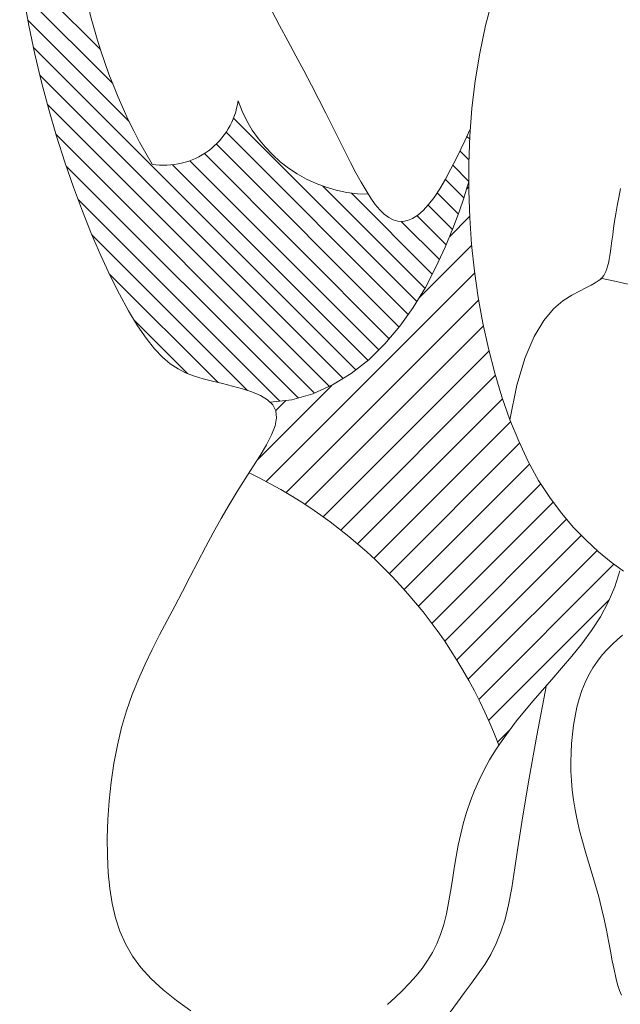
# Model space of a CAD drawing. Units: inches. Extents: x -17 to 1735, y -531 to 60.
# Tile 8 of 27: x 1734.671729 to 1734.673629, y -150.221388 to -150.218274. Entities that reach past the tile are written whole.
import ezdxf

# ---------------------------------------------------------------- set-up
doc = ezdxf.new("R2010")
doc.units = ezdxf.units.IN
doc.header["$MEASUREMENT"] = 0
doc.layers.add('A-FURN', color=242, linetype='Continuous', lineweight=18, true_color=0xcd2027)

# ---------------------------------------------------------------- blocks, each defined once
blk = doc.blocks.new('childrens_room_2')
for p, q in [((70.08834575234098, 54.10698021353749), (70.08185483306764, 54.11347113283994)), ((70.08930673154421, 54.10429042615437), (70.08214777633432, 54.11144938138608)), ((70.08258798463388, 54.10893278750013), (70.08217230242329, 54.11128011434488)), ((70.11988434807748, 54.11121103807676), (70.11928737653537, 54.10893150579653)), ((70.10208583985107, 54.11016166533085), (70.10273900536006, 54.10891733597094)), ((70.0906485886185, 54.10121976091471), (70.08251318732394, 54.10935516215835)), ((70.08306719829444, 54.10662777216789), (70.08258798463388, 54.10893278750013)), ((70.10273900536006, 54.10891733597094), (70.1033990907122, 54.10769144112276)), ((70.11928737653537, 54.10893150579653), (70.11881939316984, 54.1066923617604)), ((70.10887354584295, 54.08126599547398), (70.08295051288908, 54.10718902840603)), ((70.1033990907122, 54.10769144112276), (70.10405456281617, 54.10648398077904)), ((70.08360320534442, 54.10437083808796), (70.08306719829444, 54.10662777216789)), ((70.10405456281617, 54.10648398077904), (70.10469388840605, 54.10529495493978)), ((70.11881939316984, 54.1066923617604), (70.11846210860998, 54.10447341183175)), ((70.10784346914036, 54.08056726393846), (70.08346719220165, 54.10494354092083)), ((70.10469388840605, 54.10529495493978), (70.10530755250832, 54.10412561178095)), ((70.0841892674903, 54.10216775501471), (70.08360320534442, 54.10437083808796)), ((70.10530755250832, 54.10412561178095), (70.10589411355207, 54.10298219213877)), ((70.11846210860998, 54.10447341183175), (70.11819980044268, 54.10225846865654)), ((70.10674630752649, 54.07993561737971), (70.0840715120535, 54.10261041284542)), ((70.09941784066498, 54.10282335800587), (70.0993978207803, 54.10284337791239)), ((70.10589411355207, 54.10298219213877), (70.10645414814238, 54.10187218504001)), ((70.08481864655506, 54.10002429269519), (70.0841892674903, 54.10216775501471)), ((70.10645414814238, 54.10187218504001), (70.10698823294254, 54.10080307951142)), ((70.11819980044268, 54.10225846865654), (70.11802701396985, 54.10004737197454)), ((70.11376654561494, 54.0867458448833), (70.09903804528177, 54.10147434520189)), ((70.10698823294254, 54.10080307951142), (70.10749694461586, 54.09978236455794)), ((70.10555079970393, 54.07940231700052), (70.0847728476033, 54.10018026907204)), ((70.08548460436171, 54.09794622087651), (70.08481864655506, 54.10002429269519)), ((70.11307666940732, 54.08570691289646), (70.09844286601177, 54.10034071627745)), ((70.11762279925054, 54.09966620707422), (70.1178864010831, 54.10023832820883)), ((70.1180167069647, 54.09978376548536), (70.11778412475135, 54.10001634771328)), ((70.1178864010831, 54.10023832820883), (70.118074405425, 54.1006538262431)), ((70.11802701396985, 54.10004737197454), (70.1179408612766, 54.09784396827894)), ((70.11235278042616, 54.08470199369043), (70.09765760974145, 54.09939716433149)), ((70.10749694461586, 54.09978236455794), (70.10798085982563, 54.09881752921359)), ((70.11729604716996, 54.09897629695336), (70.11762279925054, 54.09966620707422)), ((70.11155901827036, 54.08376694762996), (70.09669325274766, 54.09863271315265)), ((70.10798085982563, 54.09881752921359), (70.10844055523515, 54.09791606249058)), ((70.11691859208398, 54.09820743196036), (70.11729604716996, 54.09897629695336)), ((70.11795165449033, 54.0981200097944), (70.11722996820347, 54.0988416960376)), ((70.08618040267496, 54.09593930932027), (70.08548460436171, 54.09794622087651)), ((70.10422052682728, 54.07900378167545), (70.08559420123812, 54.09763010723549)), ((70.10983944662033, 54.08202890289834), (70.09413392528543, 54.09773442420413)), ((70.11072027858928, 54.08287687909473), (70.09553577746149, 54.09806138022253)), ((70.10844055523515, 54.09791606249058), (70.10887660750771, 54.0970854534084)), ((70.11650288117701, 54.09739844620202), (70.11691859208398, 54.09820743196036)), ((70.11793927983265, 54.09640357623579), (70.11665275362203, 54.09769010243912)), ((70.1179408612766, 54.09784396827894), (70.11793845473906, 54.09565210409204)), ((70.10887660750771, 54.0970854534084), (70.10929016996991, 54.09633203883863)), ((70.11606136174989, 54.09658817380699), (70.11650288117701, 54.09739844620202)), ((70.10929016996991, 54.09633203883863), (70.10968470260153, 54.09565754700309)), ((70.11560648104526, 54.09581544887481), (70.11606136174989, 54.09658817380699)), ((70.11754243845238, 54.09507160942888), (70.11604821205722, 54.09656583583132)), ((70.11793922599057, 54.09635456403197), (70.11779819942197, 54.09588022690008)), ((70.08689930331778, 54.09401060992826), (70.08618040267496, 54.09593930932027)), ((70.11441734911524, 54.08782384955561), (70.106220925994, 54.09602027270597)), ((70.11501391657978, 54.08895609029281), (70.10850567942137, 54.09546432743667)), ((70.10968470260153, 54.09565754700309), (70.11006424204562, 54.09506255399032)), ((70.11515068624752, 54.09511910551959), (70.11560648104526, 54.09581544887481)), ((70.11709852587549, 54.09378671381858), (70.11539416219924, 54.09549107745846)), ((70.11779819942197, 54.09588022690008), (70.11753767607618, 54.09505655266406)), ((70.11777364987532, 54.0958026108114), (70.11793880130747, 54.09596776225811)), ((70.11793845473906, 54.09565210409204), (70.11801690650057, 54.09347562589977)), ((70.1301482338563, 54.09583144119682), (70.12999662443647, 54.09511539372619)), ((70.10274766078103, 54.07874783951996), (70.08655132895686, 54.09494417134414)), ((70.11006424204562, 54.09506255399032), (70.1104328248289, 54.09454763587422)), ((70.1104328248289, 54.09454763587422), (70.11079448776903, 54.09411336873603)), ((70.11426916277154, 54.094053744468), (70.11470430205694, 54.09453083342526)), ((70.11662620574819, 54.09253022573688), (70.11466675968725, 54.09448967177599)), ((70.11470430205694, 54.09453083342526), (70.11515068624752, 54.09511910551959)), ((70.11753767607618, 54.09505655266406), (70.11715804838926, 54.0939461216389)), ((70.12999662443647, 54.09511539372619), (70.12986671611318, 54.09443683829744)), ((70.08763456811315, 54.09217230329381), (70.08689930331778, 54.09401060992826)), ((70.11079448776903, 54.09411336873603), (70.11115326739267, 54.09376032865697)), ((70.11115326739267, 54.09376032865697), (70.1115132003429, 54.09348909171098)), ((70.11343146547327, 54.09341698579959), (70.11384498003056, 54.09368380610835)), ((70.11384498003056, 54.09368380610835), (70.11426916277154, 54.094053744468)), ((70.11715804838926, 54.0939461216389), (70.11665970868083, 54.09261151413961)), ((70.12975570048323, 54.09379654006483), (70.12966076914338, 54.09319526417533)), ((70.12986671611318, 54.09443683829744), (70.12975570048323, 54.09379654006483)), ((70.1115132003429, 54.09348909171098), (70.1118783232628, 54.09330023397927)), ((70.1118783232628, 54.09330023397927), (70.11225204811083, 54.09319490761703)), ((70.11225204811083, 54.09319490761703), (70.11263528787416, 54.09317656910428)), ((70.11558285554523, 54.09011595952183), (70.11253988749698, 54.09315892757735)), ((70.11263528787416, 54.09317656910428), (70.11302833085531, 54.0932492509732)), ((70.11302833085531, 54.0932492509732), (70.11343146547327, 54.09341698579959)), ((70.11612163642306, 54.09130598684573), (70.11378349219333, 54.09364413108272)), ((70.11638447265025, 54.09194370757035), (70.11801340944251, 54.09357264436988)), ((70.11801690650057, 54.09347562589977), (70.11817332870444, 54.09131838022443)), ((70.12966076914338, 54.09319526417533), (70.12957911374863, 54.09263377577594)), ((70.08837945888402, 54.09043785216494), (70.08763456811315, 54.09217230329381)), ((70.1001495324995, 54.07961715961431), (70.08766481304659, 54.09210187905268)), ((70.11665970868083, 54.09261151413961), (70.11604304927053, 54.09111531046659)), ((70.12950792589575, 54.09211284002089), (70.12944439723972, 54.09163322204989)), ((70.12957911374863, 54.09263377577594), (70.12950792589575, 54.09211284002089)), ((70.11817332870444, 54.09131838022443), (70.11840483366862, 54.08918421355924)), ((70.12944439723972, 54.09163322204989), (70.12938571937732, 54.09119568702448)), ((70.11393444037415, 54.08702394930736), (70.11817876413582, 54.09126827305448)), ((70.11604304927053, 54.09111531046659), (70.115308462478, 54.08952009093486)), ((70.12932933926234, 54.0908004049765), (70.12927372504376, 54.09044516548459)), ((70.12938571937732, 54.09119568702448), (70.12932933926234, 54.0908004049765)), ((70.08912723745337, 54.08882071929696), (70.08837945888402, 54.09043785216494)), ((70.12915968820337, 54.08984359206664), (70.12909871253535, 54.08959164707488)), ((70.12921760022758, 54.0901271630268), (70.12915968820337, 54.08984359206664)), ((70.12927372504376, 54.09044516548459), (70.12921760022758, 54.0901271630268)), ((70.0977938393585, 54.08024404456813), (70.08904988628231, 54.08898799764433)), ((70.10167231330298, 54.07229209627115), (70.11842493766336, 54.08904472059515)), ((70.115308462478, 54.08952009093486), (70.11445634062287, 54.0878884358521)), ((70.11840483366862, 54.08918421355924), (70.11870853347821, 54.08707697241192)), ((70.12888463820448, 54.08899751263238), (70.12879664265668, 54.08884299603818)), ((70.12896246405901, 54.08917141289425), (70.12888463820448, 54.08899751263238)), ((70.1290333966713, 54.08936852252958), (70.12896246405901, 54.08917141289425)), ((70.12909871253535, 54.08959164707488), (70.1290333966713, 54.08936852252958)), ((70.08987116564415, 54.08733436743062), (70.08912723745337, 54.08882071929696)), ((70.1280974439683, 54.08825043450491), (70.12776946056286, 54.08806403692)), ((70.12835087797023, 54.08841260252524), (70.1280974439683, 54.08825043450491)), ((70.12854303845555, 54.08855946766419), (70.12835087797023, 54.08841260252524)), ((70.12868720136933, 54.08869995660501), (70.12854303845555, 54.08855946766419)), ((70.12879664265668, 54.08884299603818), (70.12868720136933, 54.08869995660501)), ((70.09060450527934, 54.0859922593358), (70.08987116564415, 54.08733436743062)), ((70.11445634062287, 54.0878884358521), (70.11348707602475, 54.08628292553334)), ((70.12683674170287, 54.0875828463308), (70.1262128378253, 54.08725917655686)), ((70.12735365175061, 54.08784448308728), (70.12683674170287, 54.0875828463308)), ((70.12776946056286, 54.08806403692), (70.12735365175061, 54.08784448308728)), ((70.10325632891502, 54.07140638584536), (70.11874183262583, 54.08689188956344)), ((70.11870853347821, 54.08707697241192), (70.11908186135, 54.08500194572702)), ((70.12550558104297, 54.08680943005896), (70.12474599568989, 54.08615853973464)), ((70.1262128378253, 54.08725917655686), (70.12550558104297, 54.08680943005896)), ((70.0913205181237, 54.08480785774594), (70.09060450527934, 54.0859922593358)), ((70.11348707602475, 54.08628292553334), (70.11240187189426, 54.08475982311796)), ((70.12474599568989, 54.08615853973464), (70.12396510610009, 54.08523143845963)), ((70.09534503247006, 54.08096404322572), (70.09104428726597, 54.08526478844436)), ((70.11908186135, 54.08500194572702), (70.11952353368864, 54.08297019219611)), ((70.12396510610009, 54.08523143845963), (70.12319393660756, 54.08395305912421)), ((70.09201246605836, 54.08379462541637), (70.0913205181237, 54.08480785774594)), ((70.10478089296842, 54.07046122392642), (70.11912467337562, 54.08480500434092)), ((70.11240187189426, 54.08475982311796), (70.11120517518023, 54.08335012305764)), ((70.09267649864663, 54.08295993482028), (70.09201246605836, 54.08379462541637)), ((70.12319393660756, 54.08395305912421), (70.12246351148816, 54.08224833462594)), ((70.09332031676198, 54.08228679722964), (70.09267649864663, 54.08295993482028)), ((70.10624785745632, 54.06945846237653), (70.11957188877162, 54.08278249373546)), ((70.11120517518023, 54.08335012305764), (70.10990224378068, 54.08207850265029)), ((70.11952353368864, 54.08297019219611), (70.12003258791404, 54.08099421292575)), ((70.09395450890182, 54.08175213365615), (70.09332031676198, 54.08228679722964)), ((70.10990224378068, 54.08207850265029), (70.1084983354772, 54.08096963918655)), ((70.12246351148816, 54.08224833462594), (70.12180485513412, 54.0800421978551)), ((70.09458966362175, 54.08133286510423), (70.09395450890182, 54.08175213365615)), ((70.09523636953557, 54.08100591256374), (70.09458966362175, 54.08133286510423)), ((70.09590521525709, 54.0807481970391), (70.09523636953557, 54.08100591256374)), ((70.0966067893419, 54.08053663953473), (70.09590521525709, 54.0807481970391)), ((70.0973516802874, 54.08034816104777), (70.0966067893419, 54.08053663953473)), ((70.09814325732762, 54.08016176609675), (70.0973516802874, 54.08034816104777)), ((70.1084983354772, 54.08096963918655), (70.10699870810961, 54.08004820996433)), ((70.10765865067836, 54.06839952964077), (70.12008374557948, 54.08082462454188)), ((70.12003258791404, 54.08099421292575), (70.12060806150433, 54.07908650905159)), ((70.09895601147903, 54.07996479327852), (70.09814325732762, 54.08016176609675)), ((70.09975721443655, 54.07974666471858), (70.09895601147903, 54.07996479327852)), ((70.10051413783688, 54.07949680254245), (70.09975721443655, 54.07974666471858)), ((70.10119405337494, 54.0792046288538), (70.10051413783688, 54.07949680254245)), ((70.10095389590018, 54.07404340484794), (70.10692648183206, 54.08001599077983)), ((70.10699870810961, 54.08004820996433), (70.1054086195177, 54.07933889226701)), ((70.12180485513412, 54.0800421978551), (70.1212489918212, 54.07725958168743)), ((70.10176423262922, 54.0788595657927), (70.10119405337494, 54.0792046288538)), ((70.10219194729464, 54.07845103545554), (70.10176423262922, 54.0788595657927)), ((70.10373332748307, 54.07886636339248), (70.10197808996193, 54.07865530062412)), ((70.10243236198906, 54.07799159690188), (70.10324887420168, 54.07880810913633)), ((70.1054086195177, 54.07933889226701), (70.10373332748307, 54.07886636339248)), ((70.10901432415588, 54.06728547708048), (70.12066189823555, 54.07893305120381)), ((70.12060806150433, 54.07908650905159), (70.1212489918212, 54.07725958168743)), ((70.1024444690079, 54.07796845998968), (70.10219194729464, 54.07845103545554)), ((70.10249901633827, 54.07740382583), (70.1024444690079, 54.07796845998968)), ((70.10237259506133, 54.07675937677272), (70.10249901633827, 54.07740382583)), ((70.1103155845299, 54.06611701147489), (70.12130948552979, 54.07711091248206)), ((70.1212489918212, 54.07725958168743), (70.12195441622637, 54.07552593196164)), ((70.10209215800162, 54.07603992094522), (70.10237259506133, 54.07675937677272)), ((70.10168465792552, 54.07525026647494), (70.10209215800162, 54.07603992094522)), ((70.12195441622637, 54.07552593196164), (70.12272337219795, 54.07389806098803)), ((70.10117704759935, 54.07439522148928), (70.10168465792552, 54.07525026647494)), ((70.11156281515608, 54.06489451612145), (70.12203135418125, 54.07536305516117)), ((70.10059627973126, 54.07347959410839), (70.10117704759935, 54.07439522148928)), ((70.12272337219795, 54.07389806098803), (70.12355489703944, 54.07238846989497)), ((70.09996930720402, 54.07250819246695), (70.10059627973126, 54.07347959410839)), ((70.11275608704776, 54.06361806201897), (70.12283444283415, 54.07369641781264)), ((70.09932308260935, 54.07148582468511), (70.09996930720402, 54.07250819246695)), ((70.12355489703944, 54.07238846989497), (70.12444610295236, 54.07100645438771)), ((70.11389516097145, 54.06228740991213), (70.12372791599367, 54.072120164978)), ((70.09867990629166, 54.07041777970738), (70.09932308260935, 54.07148582468511)), ((70.12444610295236, 54.07100645438771), (70.12538640143933, 54.06974848850808)), ((70.098043468151, 54.06931126971762), (70.09867990629166, 54.07041777970738)), ((70.1149794804037, 54.06090200335751), (70.12471893145587, 54.07064145442422)), ((70.09741280554911, 54.06817398772403), (70.098043468151, 54.06931126971762)), ((70.11600815534942, 54.05946095233088), (70.1258058840281, 54.06925868100228)), ((70.12538640143933, 54.06974848850808), (70.12636327866815, 54.06860784087479)), ((70.12636327866815, 54.06860784087479), (70.12736422086485, 54.0675777801211)), ((70.09678695596406, 54.06701362673487), (70.09741280554911, 54.06817398772403)), ((70.11697993521696, 54.05796300616788), (70.1269849812484, 54.06796805224297)), ((70.12736422086485, 54.0675777801211), (70.12837671419723, 54.06665157487299)), ((70.09616495675758, 54.06583787974381), (70.09678695596406, 54.06701362673487)), ((70.11789316894604, 54.0564065139319), (70.12825216476224, 54.06676550976266)), ((70.12837671419723, 54.06665157487299), (70.12938824494952, 54.06582249374918)), ((70.09554584534956, 54.06465443976634), (70.09616495675758, 54.06583787974381)), ((70.11874575017603, 54.05478936917501), (70.12961272826536, 54.06565634724251)), ((70.12938824494952, 54.06582249374918), (70.13038629923133, 54.06508380538292)), ((70.09492865915993, 54.06347099979615), (70.09554584534956, 54.06465443976634)), ((70.12968858571142, 54.06382724418512), (70.13009287324851, 54.0651205886083)), ((70.12915599091096, 54.06259928474759), (70.12968858571142, 54.06382724418512)), ((70.09431243555039, 54.06229525284874), (70.09492865915993, 54.06347099979615)), ((70.1195350413432, 54.05310893431163), (70.12925601961209, 54.06282991257325)), ((70.09369765584009, 54.06113184676946), (70.09431243555039, 54.06229525284874)), ((70.12851902028663, 54.06143296576778), (70.12915599091096, 54.06259928474759)), ((70.12780160527792, 54.06032454273958), (70.12851902028663, 54.06143296576778)), ((70.09309057688691, 54.05997324883941), (70.09369765584009, 54.06113184676946)), ((70.09249889956439, 54.05880888116229), (70.09309057688691, 54.05997324883941)), ((70.1270276774408, 54.05927027113506), (70.12780160527792, 54.06032454273958)), ((70.12990142278025, 54.05961865505236), (70.13030191418832, 54.0599567170488)), ((70.1262211682147, 54.05826640644085), (70.1270276774408, 54.05927027113506)), ((70.12907795015374, 54.05882213063745), (70.12949055143284, 54.05924026755241)), ((70.12949055143284, 54.05924026755241), (70.12990142278025, 54.05961865505236)), ((70.09193032457145, 54.05762816587088), (70.09249889956439, 54.05880888116229)), ((70.12540600892274, 54.05730920412901), (70.1262211682147, 54.05826640644085)), ((70.12828215724906, 54.05786891287283), (70.12867226871779, 54.0583648203887)), ((70.12867226871779, 54.0583648203887), (70.12907795015374, 54.05882213063745)), ((70.09139255278163, 54.05642052508341), (70.09193032457145, 54.05762816587088)), ((70.12460613123724, 54.05639491968617), (70.12540600892274, 54.05730920412901)), ((70.12758324342897, 54.05676361037189), (70.12791626546417, 54.05733498417106)), ((70.12791626546417, 54.05733498417106), (70.12828215724906, 54.05786891287283)), ((70.12728991488578, 54.05615603963673), (70.12758324342897, 54.05676361037189)), ((70.09089328495205, 54.05517538091084), (70.09139255278163, 54.05642052508341)), ((70.12418785965886, 54.05597707063719), (70.12340028398788, 54.05189968368944)), ((70.12384152588086, 54.05551932852398), (70.12460613123724, 54.05639491968617)), ((70.12703579938855, 54.05551620850605), (70.12728991488578, 54.05615603963673)), ((70.09044022189804, 54.05388215547867), (70.09089328495205, 54.05517538091084)), ((70.123116421873, 54.05467628580521), (70.12384152588086, 54.05551932852398)), ((70.12681859016769, 54.05484872560776), (70.12703579938855, 54.05551620850605)), ((70.12243110751618, 54.05385916662493), (70.123116421873, 54.05467628580521)), ((70.12648566417514, 54.05344923902015), (70.12663598062821, 54.05415819956982)), ((70.12663598062821, 54.05415819956982), (70.12681859016769, 54.05484872560776)), ((70.09004106437672, 54.05253027091243), (70.09044022189804, 54.05388215547867)), ((70.12178587111296, 54.05306134607093), (70.12243110751618, 54.05385916662493)), ((70.12636533403887, 54.05272645257941), (70.12648566417514, 54.05344923902015)), ((70.12118100096589, 54.05227619923102), (70.12178587111296, 54.05306134607093)), ((70.12627268374084, 54.05199444889007), (70.12636533403887, 54.05272645257941)), ((70.0897020693042, 54.05111411772526), (70.09004106437672, 54.05253027091243)), ((70.12025777088596, 54.05136193791844), (70.12121109322062, 54.05231526020947)), ((70.12061678549392, 54.05149710120753), (70.12118100096589, 54.05227619923102)), ((70.12340028398788, 54.05189968368944), (70.12278657174787, 54.04846577627035)), ((70.12620540645324, 54.0512578365728), (70.12627268374084, 54.05199444889007)), ((70.0894237179414, 54.04964796002463), (70.0897020693042, 54.05111411772526)), ((70.12009351305781, 54.05071742709555), (70.12061678549392, 54.05149710120753)), ((70.12616186846165, 54.05051997607955), (70.12620540645324, 54.0512578365728)), ((70.11961147190189, 54.04993055197559), (70.12009351305781, 54.05071742709555)), ((70.1261431268754, 54.04977923519476), (70.12616186846165, 54.05051997607955)), ((70.08920504770823, 54.04815103030563), (70.0894237179414, 54.04964796002463)), ((70.11917061394664, 54.04913085909214), (70.11961147190189, 54.04993055197559)), ((70.12615091168439, 54.04903273353415), (70.1261431268754, 54.04977923519476)), ((70.11876954575885, 54.04831676422185), (70.11917061394664, 54.04913085909214)), ((70.1261869529367, 54.04827759069161), (70.12615091168439, 54.04903273353415)), ((70.08904509602465, 54.04664256108521), (70.08920504770823, 54.04815103030563)), ((70.11840653717402, 54.04748769130532), (70.11876954575885, 54.04831676422185)), ((70.12278657174787, 54.04846577627035), (70.1223129882815, 54.04559988214026)), ((70.12625298062224, 54.04751092628288), (70.1261869529367, 54.04827759069161)), ((70.11807985831868, 54.04664306426861), (70.11840653717402, 54.04748769130532)), ((70.12635072467268, 54.04672985991641), (70.12625298062224, 54.04751092628288)), ((70.0889429002523, 54.04514178485118), (70.08904509602465, 54.04664256108521)), ((70.11778777920293, 54.04578230702322), (70.11807985831868, 54.04664306426861)), ((70.1264819150779, 54.04593151120065), (70.12635072467268, 54.04672985991641)), ((70.11752856977867, 54.04490484351703), (70.11778777920293, 54.04578230702322)), ((70.1223129882815, 54.04559988214026), (70.12194579887321, 54.04322653502316)), ((70.12664828182781, 54.04511299973677), (70.1264819150779, 54.04593151120065)), ((70.08889749775292, 54.04366793411321), (70.0889429002523, 54.04514178485118)), ((70.11730050005602, 54.04401009766883), (70.11752856977867, 54.04490484351703)), ((70.12684992108144, 54.04427250128941), (70.12664828182781, 54.04511299973677)), ((70.11710184010329, 54.0430974933974), (70.11730050005602, 54.04401009766883)), ((70.12708039338352, 54.04341241617515), (70.12684992108144, 54.04427250128941)), ((70.08890792594642, 54.04224024138096), (70.08889749775292, 54.04366793411321)), ((70.1169295144023, 54.04216808686618), (70.11710184010329, 54.0430974933974)), ((70.12194579887321, 54.04322653502316), (70.12165126880748, 54.04127026865757)), ((70.12733162556427, 54.04253620087406), (70.12708039338352, 54.04341241617515)), ((70.12759554427933, 54.04164731184431), (70.12733162556427, 54.04253620087406)), ((70.08897322225269, 54.04087793914953), (70.08890792594642, 54.04224024138096)), ((70.1167750652053, 54.04122946309366), (70.1169295144023, 54.04216808686618)), ((70.12786407630077, 54.04074920556599), (70.12759554427933, 54.04164731184431)), ((70.08909450961394, 54.03959577233621), (70.08897322225269, 54.04087793914953)), ((70.11662868923625, 54.04029083934296), (70.1167750652053, 54.04122946309366)), ((70.12165126880748, 54.04127026865757), (70.12139566342697, 54.039655616782)), ((70.12812914840063, 54.03984533849729), (70.12786407630077, 54.04074920556599)), ((70.11648058333552, 54.03936143284813), (70.11662868923625, 54.04029083934296)), ((70.08928125370178, 54.03839053553241), (70.08909450961394, 54.03959577233621)), ((70.11632094416885, 54.03845046086502), (70.11648058333552, 54.03936143284813)), ((70.12139566342697, 54.039655616782), (70.12114524801612, 54.03830711313498)), ((70.12838268729277, 54.03893916712553), (70.12812914840063, 54.03984533849729)), ((70.08954500559369, 54.03725453572992), (70.08928125370178, 54.03839053553241)), ((70.11613996851841, 54.03756714064951), (70.11632094416885, 54.03845046086502)), ((70.12114524801612, 54.03830711313498), (70.1208662879176, 54.03714929145502)), ((70.12861661969103, 54.03803414791622), (70.12838268729277, 54.03893916712553)), ((70.11592785316635, 54.03672068943563), (70.11613996851841, 54.03756714064951)), ((70.12882498676073, 54.03713498550354), (70.12861661969103, 54.03803414791622)), ((70.08989731654177, 54.03618007993504), (70.08954500559369, 54.03725453572992)), ((70.11567479489489, 54.03592032449381), (70.11592785316635, 54.03672068943563)), ((70.1208662879176, 54.03714929145502), (70.12053182413686, 54.03611604675683)), ((70.12901028747322, 54.03625137721104), (70.12882498676073, 54.03713498550354)), ((70.0903497377981, 54.03515947514683), (70.08989731654177, 54.03618007993504)), ((70.12053182413686, 54.03611604675683), (70.12014200085426, 54.03517871913066)), ((70.1291771349602, 54.03539426853098), (70.12901028747322, 54.03625137721104)), ((70.09091382044019, 54.03418502836434), (70.0903497377981, 54.03515947514683)), ((70.11502278288711, 54.0344724473602), (70.11537300866215, 54.03517247868006)), ((70.11537300866215, 54.03517247868006), (70.11567479489489, 54.03592032449381)), ((70.12014200085426, 54.03517871913066), (70.11970373802934, 54.03431800994297)), ((70.12933014252806, 54.03457460494831), (70.1291771349602, 54.03539426853098)), ((70.11462642416475, 54.03381274151474), (70.11502278288711, 54.0344724473602)), ((70.12947392359959, 54.03380333196259), (70.12933014252806, 54.03457460494831)), ((70.09160111572012, 54.0332490465866), (70.09091382044019, 54.03418502836434)), ((70.11418623920648, 54.03318587213147), (70.11462642416475, 54.03381274151474)), ((70.11970373802934, 54.03431800994297), (70.11922395556351, 54.03351462057475)), ((70.12961309130654, 54.03309139505148), (70.12947392359959, 54.03380333196259)), ((70.0924231748318, 54.03234383681996), (70.09160111572012, 54.0332490465866)), ((70.11370453460725, 54.03258435019091), (70.11418623920648, 54.03318587213147)), ((70.11922395556351, 54.03351462057475), (70.11870957341628, 54.03274925239969)), ((70.12975225901349, 54.03244973972181), (70.12961309130654, 54.03309139505148)), ((70.09338400863228, 54.03146378957029), (70.0924231748318, 54.03234383681996)), ((70.1126257929823, 54.03142739255276), (70.11318361696206, 54.03200068666632)), ((70.11318361696206, 54.03200068666632), (70.11370453460725, 54.03258435019091)), ((70.11816751143081, 54.03200260677698), (70.11760468968308, 54.03125538508033)), ((70.11870957341628, 54.03274925239969), (70.11816751143081, 54.03200260677698)), ((70.1298960400268, 54.03188931144399), (70.12975225901349, 54.03244973972181)), ((70.09445746645682, 54.03061162945817), (70.09338400863228, 54.03146378957029)), ((70.11203336932115, 54.03085697882346), (70.1126257929823, 54.03142739255276)), ((70.11760468968308, 54.03125538508033), (70.11702802801622, 54.03048828868344)), ((70.13004914369552, 54.03141865540096), (70.1298960400268, 54.03188931144399)), ((70.13021666388843, 54.03103671543653), (70.13004914369552, 54.03141865540096)), ((70.09560985742021, 54.02979216459647), (70.09445746645682, 54.03061162945817)), ((70.11141095916858, 54.03028320464222), (70.11203336932115, 54.03085697882346)), ((70.11702802801622, 54.03048828868344), (70.11644430215122, 54.02968633954009))]:
    blk.add_line(p, q)
for centre, radius, start, end in [((70.13126567467, 54.1207976377322), 0.0450892553131211, 131.1239089098638, 210.6911252888027), ((70.09348998324597, 54.10366414034655), 0.005964578347911, 260.3681689528154, 352.3451692867589), ((70.11000777165057, 54.10661020368428), 0.0112466367544215, 199.4263532438815, 269.3680232654616), ((70.25073743193526, 54.66704331015939), 0.5911939097029936, 258.0690127884769, 260.1371981708295), ((70.0829508595157, 54.03695112298596), 0.0399934647922624, 20.7298019305562, 64.3184341249087)]:
    blk.add_arc(centre, radius, start, end)

msp = doc.modelspace()

# ---------------------------------------------------------------- block references
at = {"layer": 'A-FURN', "xscale": 0.0393700787401575, "yscale": 0.0393700787401575, "zscale": 0.0393700787401575}
msp.add_blockref('childrens_room_2', (1731.912600860487, -152.3485650223338), dxfattribs=at)

doc.saveas('drawing.dxf')
